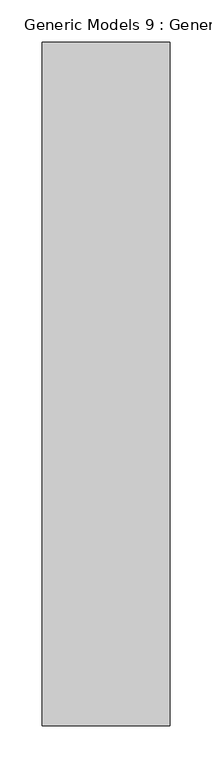
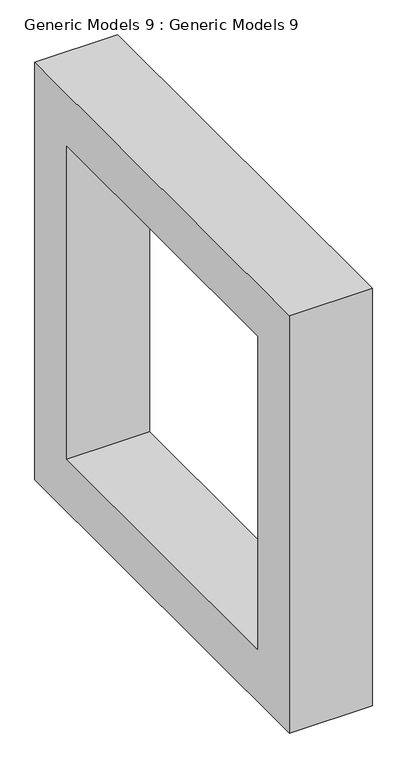
"""IFC4 building model written with IfcOpenShell, lengths in millimetres: proxy geometry, Generic Models 9 : Generic Models 9."""

from ifc_helpers import new_model, si_unit, frame, origin, place, context, project, spatial, polyline, outline, extrude, source, transform, mapped, element, save


def generic_models_9_generic_models_9_c35f1afa(model_context):
    return source(origin(), model_context, "Body", "SweptSolid", [
        extrude(outline(polyline([(7048.5641252, 9339.5849297), (7861.3641252, 9339.5849297), (7861.3641252, 8526.7849297), (7048.5641252, 8526.7849297), (7048.5641252, 9339.5849297)]), holes=[polyline([(7150.1641252, 9237.9849297), (7150.1641252, 8628.3849297), (7759.7641252, 8628.3849297), (7759.7641252, 9237.9849297), (7150.1641252, 9237.9849297)])]), frame((-6249.8280307, 0.0, 0.0), z_axis=(1.0, 0.0, 0.0), x_axis=(0.0, 1.0, 0.0)), (0.0, 0.0, 1.0), 152.4),
    ])


if __name__ == "__main__":
    model = new_model("IFC4")
    model_context = context("Model", 3, world=origin())
    ifc_project = project(units=[si_unit("LENGTHUNIT", "METRE", prefix="MILLI")], contexts=[model_context])
    site = spatial("IfcSite", under=ifc_project)
    building = spatial("IfcBuilding", under=site)
    placement = place(None, origin())
    generic_models_9_generic_models_9_shape = generic_models_9_generic_models_9_c35f1afa(model_context)
    element("IfcBuildingElementProxy", 1, Name="Generic Models 9 : Generic Models 9", ObjectType="Generic Models 9 : Generic Models 9", at=placement, inside=building, context=model_context, shape_type="MappedRepresentation", body=[
        mapped(generic_models_9_generic_models_9_shape, transform((0.0, 0.0, 0.0), x_axis=(1.0, 0.0, 0.0), y_axis=(0.0, 1.0, 0.0), z_axis=(0.0, 0.0, 1.0))),
    ])
    save(model, "model.ifc")

# Revit data of these elements
# Element 1 (IfcBuildingElementProxy, "Generic Models 9 : Generic Models 9")
#   Materials on its faces: "chocolate brown"
# Materials
#   "chocolate brown": class "Generic", colour RGB 120 120 120, transparency 0, Cost = 0
